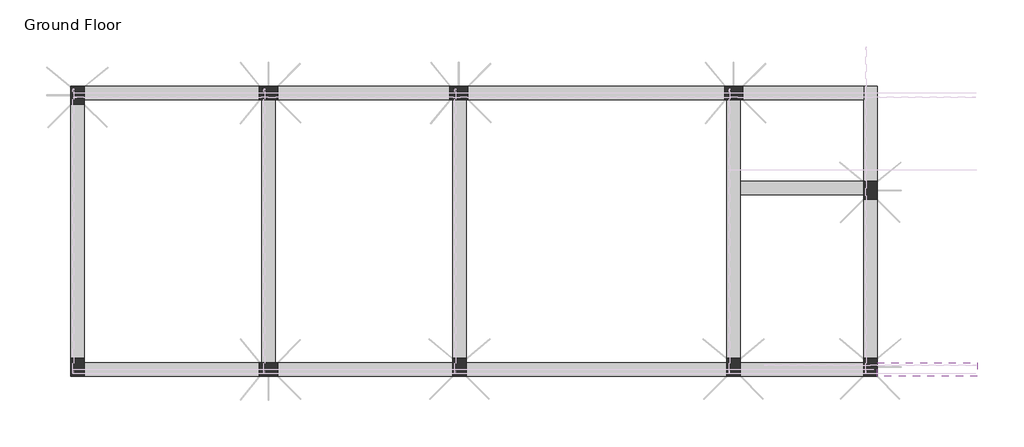
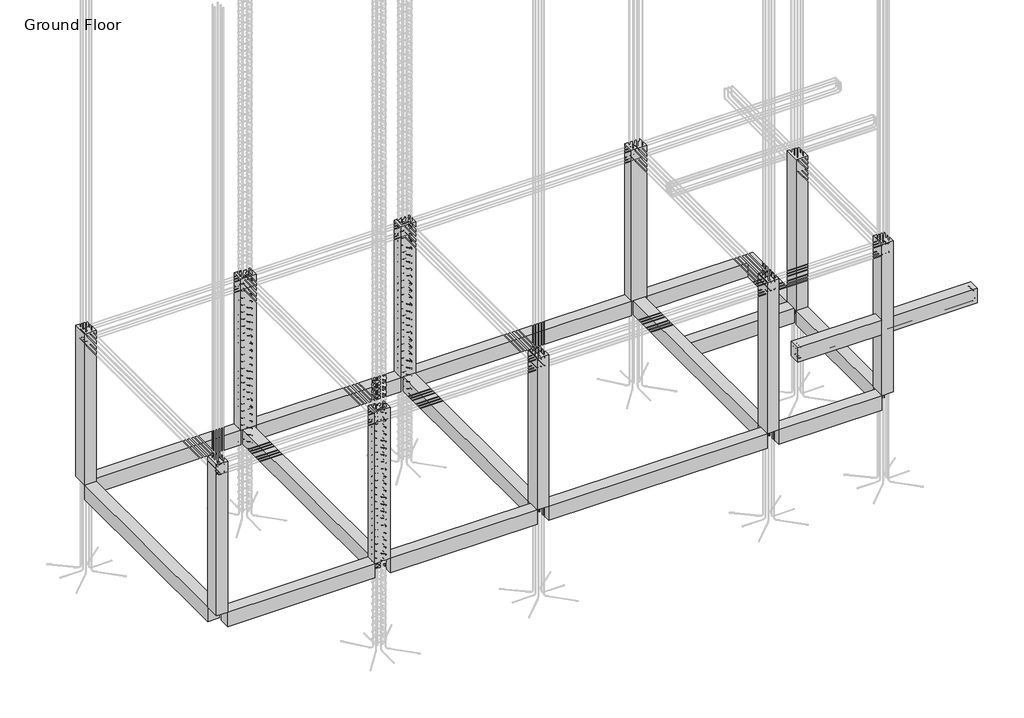
# One storey, part 1 of 5: 10 columns, 9 beams.
"""IFC4 building model written with IfcOpenShell, lengths in millimetres."""

from ifc_helpers import new_model, si_unit, frame, origin, origin_with_axes, place, context, project, spatial, polyline, outline, extrude, faceted_brep, element, save

model = new_model("IFC4")

# Units and contexts
model_context = context("Model", 3, world=origin())
ifc_project = project(units=[si_unit("LENGTHUNIT", "METRE", prefix="MILLI")], contexts=[model_context])

# Site, building, storey
site = spatial("IfcSite", under=ifc_project)
building = spatial("IfcBuilding", under=site)
storey = spatial("IfcBuildingStorey", under=building, Name="Ground Floor", Elevation=0.0)

# Beams
placement = place(None, origin())
element("IfcBeam", 1, ObjectType="M_Concrete-Rectangular Beam : 9\" X12\"", at=placement, inside=storey, context=model_context, shape_type="SweptSolid", body=[
    extrude(outline(polyline([(3956.0882476, 415.0334631), (3956.0882476, 186.4334631), (1885.9882476, 186.4334631), (1885.9882476, 415.0334631), (3956.0882476, 415.0334631)])), frame((0.0, 0.0, -304.8), z_axis=(0.0, 0.0, 1.0), x_axis=(1.0, 0.0, 0.0)), (0.0, 0.0, 1.0), 304.8),
    extrude(outline(polyline([(-9150.3117524, 186.4334631), (-9150.3117524, 415.0334631), (-6203.9117524, 415.0334631), (-6203.9117524, 186.4334631), (-9150.3117524, 186.4334631)])), frame((0.0, 0.0, -304.8), z_axis=(0.0, 0.0, 1.0), x_axis=(1.0, 0.0, 0.0)), (0.0, 0.0, 1.0), 304.8),
    extrude(outline(polyline([(-5899.1117524, 186.4334631), (-5899.1117524, 415.0334631), (-2952.7117524, 415.0334631), (-2952.7117524, 186.4334631), (-5899.1117524, 186.4334631)])), frame((0.0, 0.0, -304.8), z_axis=(0.0, 0.0, 1.0), x_axis=(1.0, 0.0, 0.0)), (0.0, 0.0, 1.0), 304.8),
    extrude(outline(polyline([(-2724.1117524, 186.4334631), (-2724.1117524, 415.0334631), (1657.3882476, 415.0334631), (1657.3882476, 186.4334631), (-2724.1117524, 186.4334631)])), frame((0.0, 0.0, -304.8), z_axis=(0.0, 0.0, 1.0), x_axis=(1.0, 0.0, 0.0)), (0.0, 0.0, 1.0), 304.8),
])
element("IfcBeam", 2, ObjectType="M_Concrete-Rectangular Beam : 9\" X12\"", at=placement, inside=storey, context=model_context, shape_type="Brep", body=[
    faceted_brep([(4184.6882476, 5063.2334631, 0.0), (3956.0882476, 5063.2334631, 0.0), (3956.0882476, 4834.6334631, 0.0), (3956.0882476, 3463.0334631, 0.0), (4184.6882476, 3463.0334631, 0.0), (4184.6882476, 5063.2334631, -304.8), (4184.6882476, 3463.0334631, -304.8), (3956.0882476, 5063.2334631, -304.8), (3956.0882476, 3463.0334631, -304.8), (3956.0882476, 4834.6334631, -304.8)], [[[0, 1, 2, 3, 4]], [[5, 0, 4, 6]], [[7, 5, 6, 8, 9]], [[1, 7, 9, 8, 3, 2]], [[4, 3, 8, 6]], [[1, 0, 5, 7]]]),
    faceted_brep([(4184.6882476, 491.2334631, 0.0), (3956.0882476, 491.2334631, 0.0), (3956.0882476, 491.2334631, -304.8), (4184.6882476, 491.2334631, -304.8), (3956.0882476, 3158.2334631, 0.0), (4184.6882476, 3158.2334631, 0.0), (4184.6882476, 3158.2334631, -304.8), (3956.0882476, 3158.2334631, -304.8)], [[[0, 1, 2, 3]], [[4, 5, 6, 7]], [[1, 0, 5, 4]], [[0, 3, 6, 5]], [[3, 2, 7, 6]], [[2, 1, 4, 7]]]),
])
element("IfcBeam", 3, ObjectType="M_Concrete-Rectangular Beam : 9\" X12\"", at=placement, inside=storey, context=model_context, shape_type="SweptSolid", body=[
    extrude(outline(polyline([(-9150.3117524, 4834.6334631), (-9150.3117524, 5063.2334631), (-6203.9117524, 5063.2334631), (-6203.9117524, 4834.6334631), (-9150.3117524, 4834.6334631)])), frame((0.0, 0.0, -304.8), z_axis=(0.0, 0.0, 1.0), x_axis=(1.0, 0.0, 0.0)), (0.0, 0.0, 1.0), 304.8),
    extrude(outline(polyline([(3956.0882476, 5063.2334631), (3956.0882476, 4834.6334631), (1924.0882476, 4834.6334631), (1924.0882476, 5063.2334631), (3956.0882476, 5063.2334631)])), frame((0.0, 0.0, -304.8), z_axis=(0.0, 0.0, 1.0), x_axis=(1.0, 0.0, 0.0)), (0.0, 0.0, 1.0), 304.8),
    extrude(outline(polyline([(1619.2882476, 5063.2334631), (1619.2882476, 4834.6334631), (-2698.7117524, 4834.6334631), (-2698.7117524, 5063.2334631), (1619.2882476, 5063.2334631)])), frame((0.0, 0.0, -304.8), z_axis=(0.0, 0.0, 1.0), x_axis=(1.0, 0.0, 0.0)), (0.0, 0.0, 1.0), 304.8),
    extrude(outline(polyline([(-3003.5117524, 5063.2334631), (-3003.5117524, 4834.6334631), (-5899.1117524, 4834.6334631), (-5899.1117524, 5063.2334631), (-3003.5117524, 5063.2334631)])), frame((0.0, 0.0, -304.8), z_axis=(0.0, 0.0, 1.0), x_axis=(1.0, 0.0, 0.0)), (0.0, 0.0, 1.0), 304.8),
])
element("IfcBeam", 4, ObjectType="M_Concrete-Rectangular Beam : 9\" X12\"", at=placement, inside=storey, context=model_context, shape_type="SweptSolid", body=[
    extrude(outline(polyline([(-9378.9117524, 4758.4334631), (-9150.3117524, 4758.4334631), (-9150.3117524, 491.2334631), (-9378.9117524, 491.2334631), (-9378.9117524, 4758.4334631)])), frame((0.0, 0.0, -304.8), z_axis=(0.0, 0.0, 1.0), x_axis=(1.0, 0.0, 0.0)), (0.0, 0.0, 1.0), 304.8),
])
element("IfcBeam", 5, ObjectType="M_Concrete-Rectangular Beam : 9\" X12\"", at=placement, inside=storey, context=model_context, shape_type="SweptSolid", body=[
    extrude(outline(polyline([(-5937.2117524, 415.0334631), (-6165.8117524, 415.0334631), (-6165.8117524, 4834.6334631), (-5937.2117524, 4834.6334631), (-5937.2117524, 415.0334631)])), frame((0.0, 0.0, -304.8), z_axis=(0.0, 0.0, 1.0), x_axis=(1.0, 0.0, 0.0)), (0.0, 0.0, 1.0), 304.8),
])
element("IfcBeam", 6, ObjectType="M_Concrete-Rectangular Beam : 9\" X12\"", at=placement, inside=storey, context=model_context, shape_type="SweptSolid", body=[
    extrude(outline(polyline([(-2724.1117524, 491.2334631), (-2952.7117524, 491.2334631), (-2952.7117524, 4834.6334631), (-2724.1117524, 4834.6334631), (-2724.1117524, 491.2334631)])), frame((0.0, 0.0, -304.8), z_axis=(0.0, 0.0, 1.0), x_axis=(1.0, 0.0, 0.0)), (0.0, 0.0, 1.0), 304.8),
])
element("IfcBeam", 7, ObjectType="M_Concrete-Rectangular Beam : 9\" X12\"", at=placement, inside=storey, context=model_context, shape_type="Brep", body=[
    faceted_brep([(1657.3882476, 491.2334631, 0.0), (1885.9882476, 491.2334631, 0.0), (1885.9882476, 3234.4334631, 0.0), (1885.9882476, 3463.0334631, 0.0), (1885.9882476, 4834.6334631, 0.0), (1657.3882476, 4834.6334631, 0.0), (1885.9882476, 491.2334631, -304.8), (1885.9882476, 3234.4334631, -304.8), (1885.9882476, 3463.0334631, -304.8), (1885.9882476, 4834.6334631, -304.8), (1657.3882476, 491.2334631, -304.8), (1657.3882476, 4834.6334631, -304.8)], [[[0, 1, 2, 3, 4, 5]], [[1, 6, 7, 8, 9, 4, 3, 2]], [[6, 10, 11, 9, 8, 7]], [[10, 0, 5, 11]], [[1, 0, 10, 6]], [[5, 4, 9, 11]]]),
])
element("IfcBeam", 8, ObjectType="M_Concrete-Rectangular Beam : 9\" X12\"", at=placement, inside=storey, context=model_context, shape_type="SweptSolid", body=[
    extrude(outline(polyline([(3956.0882476, 3463.0334631), (3956.0882476, 3234.4334631), (1885.9882476, 3234.4334631), (1885.9882476, 3463.0334631), (3956.0882476, 3463.0334631)])), frame((0.0, 0.0, -304.8), z_axis=(0.0, 0.0, 1.0), x_axis=(1.0, 0.0, 0.0)), (0.0, 0.0, 1.0), 304.8),
])
element("IfcBeam", 9, ObjectType="M_Concrete-Rectangular Beam : 9\" X12\"", at=placement, inside=storey, context=model_context, shape_type="SweptSolid", body=[
    extrude(outline(polyline([(2271.6882476, 186.4334631), (2271.6882476, 415.0334631), (3956.0882476, 415.0334631), (3956.0882476, 186.4334631), (2271.6882476, 186.4334631)])), frame((0.0, 0.0, 1295.4), z_axis=(0.0, 0.0, 1.0), x_axis=(1.0, 0.0, 0.0)), (0.0, 0.0, 1.0), 304.8),
    extrude(outline(polyline([(5871.6882476, 415.0334631), (5871.6882476, 186.4334631), (4184.6882476, 186.4334631), (4184.6882476, 415.0334631), (5871.6882476, 415.0334631)])), frame((0.0, 0.0, 1295.4), z_axis=(0.0, 0.0, 1.0), x_axis=(1.0, 0.0, 0.0)), (0.0, 0.0, 1.0), 304.8),
])

# Columns
element("IfcColumn", 10, ObjectType="M_Concrete-Rectangular-Column : 9\" x 12\"", at=placement, inside=storey, context=model_context, shape_type="SweptSolid", body=[
    extrude(outline(polyline([(-9150.3117524, 5063.2334631), (-9150.3117524, 4758.4334631), (-9378.9117524, 4758.4334631), (-9378.9117524, 5063.2334631), (-9150.3117524, 5063.2334631)])), origin_with_axes(), (0.0, 0.0, 1.0), 3200.4),
])
element("IfcColumn", 11, ObjectType="M_Concrete-Rectangular-Column : 9\" x 12\"", at=placement, inside=storey, context=model_context, shape_type="SweptSolid", body=[
    extrude(outline(polyline([(-9150.3117524, 491.2334631), (-9150.3117524, 186.4334631), (-9378.9117524, 186.4334631), (-9378.9117524, 491.2334631), (-9150.3117524, 491.2334631)])), origin_with_axes(), (0.0, 0.0, 1.0), 3200.4),
])
element("IfcColumn", 12, ObjectType="M_Concrete-Rectangular-Column : 9\" x 12\"", at=placement, inside=storey, context=model_context, shape_type="Brep", body=[
    faceted_brep([(-6203.9117524, 415.0334631, 0.0), (-5899.1117524, 415.0334631, 0.0), (-5899.1117524, 186.4334631, 0.0), (-6203.9117524, 186.4334631, 0.0), (-6203.9117524, 415.0334631, 3200.4), (-5899.1117524, 415.0334631, 3200.4), (-5899.1117524, 415.0334631, 2895.6), (-6203.9117524, 415.0334631, 2895.6), (-5899.1117524, 186.4334631, 3200.4), (-5899.1117524, 186.4334631, 2895.6), (-6203.9117524, 186.4334631, 3200.4), (-6203.9117524, 186.4334631, 2895.6)], [[[0, 1, 2, 3]], [[4, 5, 6, 1, 0, 7]], [[5, 8, 9, 2, 1, 6]], [[8, 10, 11, 3, 2, 9]], [[10, 4, 7, 0, 3, 11]], [[4, 10, 8, 5]]]),
])
element("IfcColumn", 13, ObjectType="M_Concrete-Rectangular-Column : 9\" x 12\"", at=placement, inside=storey, context=model_context, shape_type="Brep", body=[
    faceted_brep([(-2952.7117524, 186.4334631, 0.0), (-2952.7117524, 491.2334631, 0.0), (-2724.1117524, 491.2334631, 0.0), (-2724.1117524, 186.4334631, 0.0), (-2952.7117524, 186.4334631, 3200.4), (-2952.7117524, 415.0334631, 3200.4), (-2952.7117524, 491.2334631, 3200.4), (-2952.7117524, 186.4334631, 2895.6), (-2724.1117524, 491.2334631, 3200.4), (-2724.1117524, 415.0334631, 3200.4), (-2724.1117524, 186.4334631, 3200.4), (-2724.1117524, 186.4334631, 2895.6)], [[[0, 1, 2, 3]], [[4, 5, 6, 1, 0, 7]], [[6, 8, 2, 1]], [[8, 9, 10, 11, 3, 2]], [[10, 4, 7, 0, 3, 11]], [[4, 10, 9, 8, 6, 5]]]),
])
element("IfcColumn", 14, ObjectType="M_Concrete-Rectangular-Column : 9\" x 12\"", at=placement, inside=storey, context=model_context, shape_type="Brep", body=[
    faceted_brep([(1657.3882476, 186.4334631, 0.0), (1657.3882476, 491.2334631, 0.0), (1885.9882476, 491.2334631, 0.0), (1885.9882476, 186.4334631, 0.0), (1657.3882476, 186.4334631, 3200.4), (1657.3882476, 415.0334631, 3200.4), (1657.3882476, 491.2334631, 3200.4), (1657.3882476, 186.4334631, 2895.6), (1885.9882476, 491.2334631, 3200.4), (1885.9882476, 415.0334631, 3200.4), (1885.9882476, 186.4334631, 3200.4), (1885.9882476, 186.4334631, 2895.6)], [[[0, 1, 2, 3]], [[4, 5, 6, 1, 0, 7]], [[6, 8, 2, 1]], [[8, 9, 10, 11, 3, 2]], [[10, 4, 7, 0, 3, 11]], [[4, 10, 9, 8, 6, 5]]]),
])
element("IfcColumn", 15, ObjectType="M_Concrete-Rectangular-Column : 9\" x 12\"", at=placement, inside=storey, context=model_context, shape_type="Brep", body=[
    faceted_brep([(3956.0882476, 186.4334631, 0.0), (3956.0882476, 491.2334631, 0.0), (4184.6882476, 491.2334631, 0.0), (4184.6882476, 186.4334631, 0.0), (3956.0882476, 186.4334631, 3200.4), (3956.0882476, 491.2334631, 3200.4), (3956.0882476, 186.4334631, 1295.4), (3956.0882476, 186.4334631, 1600.2), (4184.6882476, 491.2334631, 3200.4), (4184.6882476, 186.4334631, 3200.4), (4184.6882476, 186.4334631, 1600.2), (4184.6882476, 186.4334631, 1295.4)], [[[0, 1, 2, 3]], [[4, 5, 1, 0, 6, 7]], [[5, 8, 2, 1]], [[8, 9, 10, 11, 3, 2]], [[9, 4, 7, 6, 0, 3, 11, 10]], [[4, 9, 8, 5]]]),
])
element("IfcColumn", 16, ObjectType="M_Concrete-Rectangular-Column : 9\" x 12\"", at=placement, inside=storey, context=model_context, shape_type="Brep", body=[
    faceted_brep([(3956.0882476, 3158.2334631, 0.0), (3956.0882476, 3463.0334631, 0.0), (4184.6882476, 3463.0334631, 0.0), (4184.6882476, 3158.2334631, 0.0), (3956.0882476, 3158.2334631, 3200.4), (3956.0882476, 3463.0334631, 3200.4), (3956.0882476, 3463.0334631, 2895.6), (3956.0882476, 3158.2334631, 2895.6), (4184.6882476, 3463.0334631, 3200.4), (4184.6882476, 3463.0334631, 2895.6), (4184.6882476, 3158.2334631, 3200.4), (4184.6882476, 3158.2334631, 2895.6)], [[[0, 1, 2, 3]], [[4, 5, 6, 1, 0, 7]], [[5, 8, 9, 2, 1, 6]], [[8, 10, 11, 3, 2, 9]], [[10, 4, 7, 0, 3, 11]], [[4, 10, 8, 5]]]),
])
element("IfcColumn", 17, ObjectType="M_Concrete-Rectangular-Column : 9\" x 12\"", at=placement, inside=storey, context=model_context, shape_type="Brep", body=[
    faceted_brep([(1924.0882476, 4834.6334631, 0.0), (1619.2882476, 4834.6334631, 0.0), (1619.2882476, 5063.2334631, 0.0), (1924.0882476, 5063.2334631, 0.0), (1924.0882476, 4834.6334631, 3200.4), (1619.2882476, 4834.6334631, 3200.4), (1619.2882476, 4834.6334631, 2895.6), (1924.0882476, 4834.6334631, 2895.6), (1619.2882476, 5063.2334631, 3200.4), (1619.2882476, 5063.2334631, 2895.6), (1924.0882476, 5063.2334631, 3200.4), (1924.0882476, 5063.2334631, 2895.6)], [[[0, 1, 2, 3]], [[4, 5, 6, 1, 0, 7]], [[5, 8, 9, 2, 1, 6]], [[8, 10, 11, 3, 2, 9]], [[10, 4, 7, 0, 3, 11]], [[4, 10, 8, 5]]]),
])
element("IfcColumn", 18, ObjectType="M_Concrete-Rectangular-Column : 9\" x 12\"", at=placement, inside=storey, context=model_context, shape_type="Brep", body=[
    faceted_brep([(-2698.7117524, 4834.6334631, 0.0), (-3003.5117524, 4834.6334631, 0.0), (-3003.5117524, 5063.2334631, 0.0), (-2698.7117524, 5063.2334631, 0.0), (-2698.7117524, 4834.6334631, 3200.4), (-3003.5117524, 4834.6334631, 3200.4), (-3003.5117524, 4834.6334631, 2895.6), (-2698.7117524, 4834.6334631, 2895.6), (-3003.5117524, 5063.2334631, 3200.4), (-3003.5117524, 5063.2334631, 2895.6), (-2698.7117524, 5063.2334631, 3200.4), (-2698.7117524, 5063.2334631, 2895.6)], [[[0, 1, 2, 3]], [[4, 5, 6, 1, 0, 7]], [[5, 8, 9, 2, 1, 6]], [[8, 10, 11, 3, 2, 9]], [[10, 4, 7, 0, 3, 11]], [[4, 10, 8, 5]]]),
])
element("IfcColumn", 19, ObjectType="M_Concrete-Rectangular-Column : 9\" x 12\"", at=placement, inside=storey, context=model_context, shape_type="Brep", body=[
    faceted_brep([(-5899.1117524, 4834.6334631, 0.0), (-6203.9117524, 4834.6334631, 0.0), (-6203.9117524, 5063.2334631, 0.0), (-5899.1117524, 5063.2334631, 0.0), (-5899.1117524, 4834.6334631, 3200.4), (-6203.9117524, 4834.6334631, 3200.4), (-6203.9117524, 4834.6334631, 2895.6), (-5899.1117524, 4834.6334631, 2895.6), (-6203.9117524, 5063.2334631, 3200.4), (-6203.9117524, 5063.2334631, 2895.6), (-5899.1117524, 5063.2334631, 3200.4), (-5899.1117524, 5063.2334631, 2895.6)], [[[0, 1, 2, 3]], [[4, 5, 6, 1, 0, 7]], [[5, 8, 9, 2, 1, 6]], [[8, 10, 11, 3, 2, 9]], [[10, 4, 7, 0, 3, 11]], [[4, 10, 8, 5]]]),
])

save(model, "model.ifc")

# Revit data of these elements
# Type "M_Concrete-Rectangular Beam : 9\" X12\""
#   Length [instance default] = 5' - 0"
#   b = 0' - 9"
#   h = 1' - 0"
#   Structural Material [instance default] = Concrete, Cast-in-Place gray
#   Assembly Code = ""
# Type "M_Concrete-Rectangular-Column : 9\" x 12\""
#   b = 0' - 9"
#   h = 1' - 0"
#   Structural Material [instance default] = Concrete, Cast-in-Place gray
# Elements 1, 2, 3, 4, 5, 6, 7, 8, 9 (IfcBeam, "M_Concrete-Rectangular Beam : 9\" X12\"")
#   Structural Material = Concrete, Cast-in-Place gray
#   Phase Created = New Construction
#   Materials on its faces: "Concrete, Cast-in-Place gray"
# Elements 10, 11, 12, 13, 14, 15, 16, 17, 18, 19 (IfcColumn, "M_Concrete-Rectangular-Column : 9\" x 12\"")
#   Structural Material = Concrete, Cast-in-Place gray
#   Phase Created = New Construction
#   Materials on its faces: "Concrete, Cast-in-Place gray"
# Materials
#   "Concrete, Cast-in-Place gray": class "Concrete", colour RGB 192 192 192, transparency 0, Description = "Cast-in-place concrete", Cost = 0
